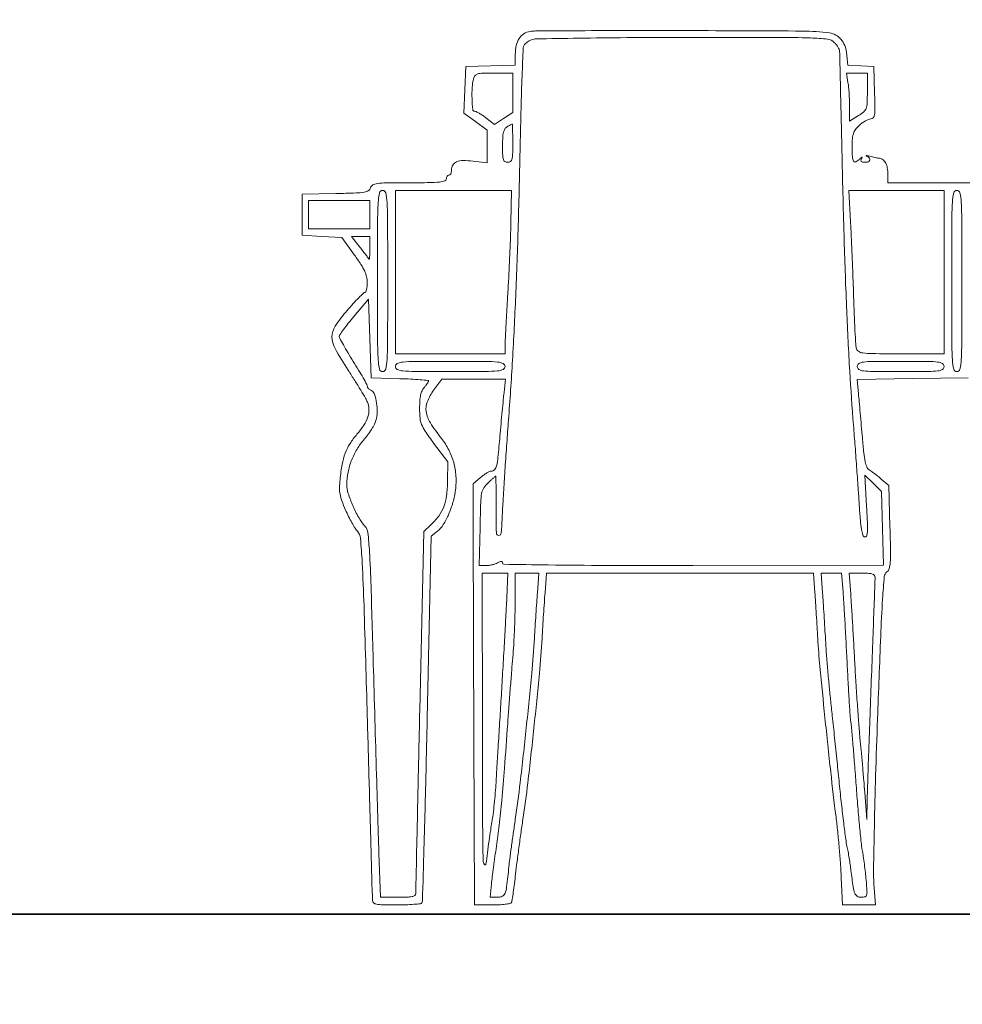
# Model space of a CAD drawing. Units: inches. Extents: x 2416 to 3391, y 1375 to 2496.
# Tile 7 of 13: x 2994 to 3014, y 2142 to 2163. Entities that reach past the tile are written whole.
import ezdxf

# ---------------------------------------------------------------- set-up
doc = ezdxf.new("R2010")
doc.units = ezdxf.units.IN
for name, color, linetype, lineweight in [('A-FLOR-PATT', 252, 'Continuous', 13), ('A-FURN', 8, 'Continuous', 18), ('A-SECT', 7, 'Continuous', 35)]:
    doc.layers.add(name, color=color, linetype=linetype, lineweight=lineweight)

msp = doc.modelspace()

# ---------------------------------------------------------------- hatches: boundary and pattern name
at = {"layer": 'A-FLOR-PATT'}
h = msp.add_hatch(dxfattribs=at)
h.set_pattern_fill('AR-CONC', color=256, scale=0.13, style=0)
h.paths.add_polyline_path([(2904.1924, 2125.8608), (3202.6924, 2125.8608), (3202.6924, 2143.8608), (2904.1924, 2143.8608)])

# ---------------------------------------------------------------- linework, layer by layer
at = {"layer": 'A-FURN'}
msp.add_lwpolyline([(3014.9326, 2159.6193), (3012.3207, 2159.6163), (3012.3199, 2159.796, 0.040694), (3012.3079, 2159.9352, 0.077699), (3012.2724, 2160.0415, 0.104071), (3012.2152, 2160.1115, 0.133976), (3012.1395, 2160.1446, -0.01143), (3012.0998, 2160.1513, -0.004315), (3012.0446, 2160.1625, -0.004271), (3011.9847, 2160.1758, -0.005193), (3011.9289, 2160.1892, 0.008277), (3011.882, 2160.2002, 0.048218), (3011.8569, 2160.2031, 0.677897), (3011.8551, 2160.1988, 0.087429), (3011.8671, 2160.1905, -0.097625), (3011.9225, 2160.1505, -0.27546), (3011.9322, 2160.1057, -0.235276), (3011.8966, 2160.0701, -0.080752), (3011.8226, 2160.0581, -0.041781), (3011.7751, 2160.0621, -0.145697), (3011.7478, 2160.0755, -0.229007), (3011.7392, 2160.0973, -0.110072), (3011.7482, 2160.1268, 0.009535), (3011.7676, 2160.1628, 0.561535), (3011.7644, 2160.1681, 0.184745), (3011.7536, 2160.1639, 0.004358), (3011.713, 2160.1268, -0.07556), (3011.6312, 2160.0712, -0.381609), (3011.5824, 2160.0853, -0.128327), (3011.5562, 2160.1691, -0.012145), (3011.5509, 2160.3858, -0.014739), (3011.5564, 2160.5722, -0.063299), (3011.5769, 2160.6811, -0.086122), (3011.6205, 2160.7643, -0.041944), (3011.7016, 2160.8532, -0.02943), (3011.7665, 2160.9066, -0.029846), (3011.837, 2160.9518, -0.03127), (3011.9028, 2160.9835, -0.096699), (3011.9509, 2160.9929, 0.227876), (3012.0031, 2161.0179, 0.132851), (3012.0314, 2161.0829, 0.039646), (3012.0407, 2161.2215, 0.003895), (3012.034, 2161.5565), (3012.0183, 2162.1201), (3011.7364, 2162.1365), (3011.4544, 2162.1529), (3011.4279, 2162.4293, 0.152427), (3011.3098, 2162.7098, 0.185846), (3011.0619, 2162.846, 0.032345), (3010.4828, 2162.8868, 0.000914), (3007.9886, 2162.8962, 0.000694), (3006.7403, 2162.897, 0.00108), (3005.6642, 2162.8938, 0.000296), (3004.7262, 2162.8884, 0.037431), (3004.6095, 2162.8789, 0.105975), (3004.4761, 2162.8276, 0.106001), (3004.3754, 2162.7261, 0.089007), (3004.3134, 2162.5763, 0.053798), (3004.2927, 2162.3848), (3004.2927, 2162.1516), (3003.7613, 2162.1358), (3003.2298, 2162.1201), (3003.2064, 2161.6185), (3003.1829, 2161.1169), (3003.4354, 2160.9356), (3003.6879, 2160.7543), (3003.6879, 2160.3998), (3003.6879, 2160.0454), (3003.3825, 2160.0836, 0.030857), (3003.166, 2160.0971, 0.100929), (3003.0261, 2160.0687, 0.165736), (3002.9473, 2159.9983, 0.128801), (3002.918, 2159.8864, -0.05129), (3002.914, 2159.8469, -0.071223), (3002.9019, 2159.8135, -0.091278), (3002.884, 2159.791, -0.181272), (3002.8631, 2159.7832, 0.148195), (3002.8421, 2159.7768, 0.098894), (3002.8242, 2159.7589, 0.082425), (3002.8122, 2159.7322, 0.064853), (3002.8081, 2159.7007, -0.329446), (3002.7755, 2159.6567, -0.048884), (3002.6606, 2159.6334, -0.022422), (3002.4464, 2159.621, -0.003188), (3002.0056, 2159.6182, 0.002574), (3001.5111, 2159.6157, 0.029876), (3001.318, 2159.6021, 0.094817), (3001.2217, 2159.5703, 0.204563), (3001.1748, 2159.5098, -0.193942), (3001.13, 2159.4495, -0.096668), (3001.0393, 2159.4157, -0.032405), (3000.8603, 2159.398, -0.003136), (3000.4239, 2159.3861), (2999.7013, 2159.3708), (2999.7013, 2158.9309), (2999.7013, 2158.491), (3000.127, 2158.4635), (3000.5526, 2158.436), (3000.828, 2158.0577, -0.011737), (3000.9673, 2157.8567, -0.036601), (3001.0475, 2157.713, -0.052571), (3001.0893, 2157.5913, -0.056553), (3001.1035, 2157.4666, -0.022205), (3001.0999, 2157.385, -0.035618), (3001.0888, 2157.3163, -0.040242), (3001.0728, 2157.2668, -0.30351), (3001.0534, 2157.2538, 0.194234), (3001.0227, 2157.2414, 0.005517), (3000.9196, 2157.1398, 0.010456), (3000.8004, 2157.0144, 0.00691), (3000.6685, 2156.8657, 0.0303), (3000.4085, 2156.5247, 0.153578), (3000.3419, 2156.2982, 0.122989), (3000.4095, 2156.0476, 0.016581), (3000.6927, 2155.5767, -0.003431), (3000.8333, 2155.3564, -0.004245), (3000.961, 2155.1492, -0.003502), (3001.0655, 2154.9737, -0.031298), (3001.1059, 2154.8936, -0.096896), (3001.139, 2154.7395, -0.083072), (3001.1146, 2154.5752, -0.06581), (3001.0295, 2154.3966, -0.034373), (3000.8811, 2154.1992, 0.037733), (3000.7308, 2153.9965, 0.050819), (3000.6292, 2153.792, 0.04407), (3000.5618, 2153.5496, 0.020527), (3000.5155, 2153.2263, 0.022179), (3000.5051, 2153.0445, 0.048115), (3000.5168, 2152.9052, 0.043671), (3000.5558, 2152.7627, 0.015462), (3000.6354, 2152.5664, 0.011422), (3000.7011, 2152.4265, 0.011589), (3000.7729, 2152.2904, 0.011437), (3000.8407, 2152.175, 0.045753), (3000.8899, 2152.1096, -0.163464), (3000.9561, 2151.9585, -0.008854), (3000.9936, 2151.432, -0.005716), (3001.0327, 2150.4986, -0.000497), (3001.1029, 2148.1231, -0.000065), (3001.1452, 2146.6311, -0.000104), (3001.1809, 2145.3591, -0.000016), (3001.2123, 2144.2298, -0.006771), (3001.2134, 2144.1532, 0.226585), (3001.2376, 2144.1026, 0.124527), (3001.3014, 2144.0733, 0.041075), (3001.4339, 2144.0599, 0.004763), (3001.7326, 2144.057, 0.008183), (3001.9336, 2144.0603, 0.012537), (3002.1075, 2144.0704, 0.007028), (3002.2511, 2144.0843, 0.230516), (3002.2798, 2144.1025, 0.131862), (3002.2918, 2144.1425, 0.000089), (3002.325, 2145.2879, 0.001058), (3002.3591, 2146.5655, 0.000646), (3002.3942, 2148.0741), (3002.4805, 2152.0003), (3002.6157, 2152.1114, 0.081242), (3002.7405, 2152.2535, 0.03703), (3002.856, 2152.4728, 0.034682), (3002.9484, 2152.7327, 0.035128), (3003.0034, 2153.0018, 0.049123), (3003.0133, 2153.2983, 0.050541), (3002.9648, 2153.5882, 0.050681), (3002.8593, 2153.8617, 0.049933), (3002.7006, 2154.1098, -0.026423), (3002.4617, 2154.4472, -0.102499), (3002.3722, 2154.6858, -0.136101), (3002.3974, 2154.9025, -0.061997), (3002.5379, 2155.1535), (3002.7076, 2155.3842), (3003.3941, 2155.3842), (3004.0807, 2155.3842), (3004.0491, 2155.0956, 0.003117), (3004.0333, 2154.9421, 0.000851), (3004.0103, 2154.6996, 0.00086), (3003.9851, 2154.4246, 0.000896), (3003.9612, 2154.1531, -0.003262), (3003.9191, 2153.6991, -0.036009), (3003.888, 2153.5194, -0.119587), (3003.8445, 2153.4359, -0.216199), (3003.7756, 2153.4047, 0.111698), (3003.7384, 2153.3963, 0.023035), (3003.6788, 2153.3644, 0.023156), (3003.6115, 2153.32, 0.019991), (3003.5452, 2153.2675), (3003.3854, 2153.1303), (3003.3854, 2152.209, 0.000667), (3003.3862, 2151.6546, 0.000091), (3003.3895, 2150.4963, 0.000105), (3003.3939, 2149.1241, 0.000088), (3003.3992, 2147.6724), (3003.4129, 2144.057), (3003.7946, 2144.057, 0.011615), (3003.9429, 2144.0605, 0.017148), (3004.0727, 2144.071, 0.012457), (3004.1776, 2144.0857, 0.216373), (3004.2056, 2144.1045, 0.097359), (3004.2192, 2144.1407, 0.003403), (3004.243, 2144.2897, 0.00622), (3004.2679, 2144.4669, 0.004297), (3004.2918, 2144.6681, -0.004039), (3004.3211, 2144.9162, -0.0018), (3004.3636, 2145.2426, -0.001782), (3004.411, 2145.5876, -0.002412), (3004.4565, 2145.8991, 0.008466), (3004.562, 2146.688, 0.002671), (3004.6933, 2147.87, 0.002626), (3004.8114, 2149.0473, 0.009341), (3004.869, 2149.8031, -0.001077), (3004.8834, 2150.0447, -0.000757), (3004.9007, 2150.3166, -0.000764), (3004.9179, 2150.5768, -0.0016), (3004.9323, 2150.7791), (3004.964, 2151.2053), (3007.8393, 2151.2053), (3010.7147, 2151.2053), (3010.7464, 2150.7791, -0.001616), (3010.7607, 2150.5768, -0.000771), (3010.778, 2150.3166, -0.000764), (3010.7952, 2150.0447, -0.001088), (3010.8096, 2149.8031, 0.009311), (3010.8559, 2149.1931, 0.001798), (3010.9643, 2148.0916, 0.002045), (3011.0886, 2146.921, 0.00359), (3011.2023, 2145.954, -0.005555), (3011.2383, 2145.6373, -0.003761), (3011.2725, 2145.2756, -0.003789), (3011.3004, 2144.9255, -0.007555), (3011.3161, 2144.6481), (3011.3407, 2144.057), (3011.6982, 2144.057), (3012.0557, 2144.057), (3012.0202, 2144.5106, -0.023542), (3012.0107, 2144.8164, -0.001398), (3012.0282, 2145.7418, -0.002102), (3012.0568, 2146.844, -0.001549), (3012.0973, 2148.0646, -0.000733), (3012.1647, 2149.8479, -0.006199), (3012.2061, 2150.6501, -0.006766), (3012.2435, 2151.1307, -0.215322), (3012.3003, 2151.2311, 0.172904), (3012.3488, 2151.3024, 0.046951), (3012.3709, 2151.439, 0.021167), (3012.3769, 2151.6806, 0.002768), (3012.3649, 2152.1946), (3012.339, 2153.0921), (3012.1739, 2153.2346, 0.007641), (3012.1039, 2153.2933, 0.006997), (3012.0301, 2153.3515, 0.007013), (3011.9628, 2153.4016, 0.02266), (3011.9161, 2153.4322, -0.164534), (3011.8671, 2153.4893, -0.043552), (3011.8315, 2153.6059, -0.025507), (3011.8012, 2153.7957, -0.005821), (3011.7702, 2154.1195, 0.000569), (3011.7476, 2154.3848, 0.000516), (3011.7236, 2154.6587, 0.000516), (3011.7017, 2154.9038, 0.001658), (3011.6863, 2155.067), (3011.6557, 2155.3821), (3012.8543, 2155.3969), (3014.0528, 2155.4117)], format="xyb", dxfattribs=at)
for points in [[(3011.166, 2162.6425, -0.026778), (3011.2084, 2162.5953, -0.028055), (3011.2447, 2162.5446, -0.029182), (3011.2709, 2162.4975, -0.099615), (3011.2796, 2162.4638, -0.007318), (3011.2816, 2162.4095, -0.000026), (3011.2963, 2161.7691, -0.000141), (3011.3127, 2161.0437, -0.000089), (3011.3315, 2160.1956, 0.001893), (3011.3785, 2158.3755, 0.00325), (3011.4332, 2156.8588, 0.003838), (3011.4987, 2155.5561, 0.005389), (3011.5786, 2154.3945, -0.00099), (3011.6142, 2153.9359, -0.000806), (3011.6505, 2153.4447, -0.000814), (3011.6826, 2152.9921, -0.002127), (3011.7037, 2152.6668, 0.005605), (3011.7267, 2152.3468, 0.021905), (3011.7517, 2152.1501, 0.031188), (3011.781, 2152.0267, 0.24354), (3011.821, 2151.9857, 0.404876), (3011.8594, 2152.0043, 0.072476), (3011.8775, 2152.0902, 0.025662), (3011.8795, 2152.2671, 0.003415), (3011.862, 2152.6403), (3011.8254, 2153.3206), (3012.0036, 2153.1424), (3012.1818, 2152.9642), (3012.2023, 2152.1698), (3012.2229, 2151.3754), (3008.1203, 2151.3716, -0.000826), (3006.2417, 2151.373, -0.002714), (3005.0015, 2151.3827, -0.000471), (3004.047, 2151.3963, -0.409789), (3004.0178, 2151.426, 0.166213), (3004.0104, 2151.4476, 0.22914), (3003.9923, 2151.4565, 0.10154), (3003.9604, 2151.4504, 0.024401), (3003.9114, 2151.4271, -0.043973), (3003.8603, 2151.4053, -0.023243), (3003.7937, 2151.3869, -0.022945), (3003.7233, 2151.3744, -0.032736), (3003.66, 2151.3702), (3003.515, 2151.3702), (3003.5327, 2152.1899, -0.002627), (3003.5472, 2152.7296, -0.036146), (3003.5676, 2152.9242, -0.096216), (3003.6129, 2153.0418, -0.065991), (3003.7044, 2153.1521, -0.003279), (3003.7643, 2153.2068, -0.005161), (3003.8164, 2153.2529, -0.00157), (3003.862, 2153.2921, -0.176898), (3003.8694, 2153.2948, -0.410724), (3003.8739, 2153.2905, -0.000294), (3003.8771, 2153.1092, -0.002699), (3003.8795, 2152.9052, -0.001618), (3003.8803, 2152.6629, 0.003665), (3003.8846, 2152.0706, 0.408936), (3003.9357, 2152.0201, 0.396408), (3003.9893, 2152.0702, 0.00365), (3004.0233, 2152.6624, -0.00305), (3004.042, 2152.996, -0.001065), (3004.0729, 2153.4757, -0.001058), (3004.1091, 2154.0035, -0.001235), (3004.1458, 2154.5045, 0.004548), (3004.2317, 2155.7945, 0.003739), (3004.3006, 2157.1729, 0.003361), (3004.355, 2158.6944, 0.002316), (3004.397, 2160.4189, -0.001849), (3004.416, 2161.2262, -0.002933), (3004.4388, 2161.9173, -0.000677), (3004.4631, 2162.5223, -0.128702), (3004.4811, 2162.581, -0.068231), (3004.5058, 2162.6109, -0.029137), (3004.546, 2162.6438, -0.028159), (3004.5936, 2162.6745, -0.033036), (3004.642, 2162.6978, -0.091686), (3004.7375, 2162.7172, -0.000531), (3005.6501, 2162.7325, -0.002226), (3006.6929, 2162.7442, -0.001411), (3007.9081, 2162.7489, -0.000515), (3009.9481, 2162.7491, -0.007931), (3010.6506, 2162.7373, -0.018651), (3011.0223, 2162.7112, -0.171176)], [(3004.237, 2161.5565), (3004.2364, 2161.1303), (3004.0403, 2161.0033), (3003.8443, 2160.8763), (3003.6598, 2161.0171, 0.014107), (3003.5848, 2161.071, 0.01763), (3003.5122, 2161.1165, 0.015997), (3003.4496, 2161.1501, 0.115683), (3003.4166, 2161.1578, -0.387752), (3003.3746, 2161.1962, -0.014242), (3003.3599, 2161.43, -0.023123), (3003.3628, 2161.6746, -0.050938), (3003.3926, 2161.8589, -0.105762), (3003.4274, 2161.9269, -0.154427), (3003.4832, 2161.9636, -0.06207), (3003.5873, 2161.9794, -0.006663), (3003.8317, 2161.9826), (3004.2377, 2161.9826)], [(3011.8785, 2161.584, -0.008054), (3011.8729, 2161.3271, -0.079294), (3011.8518, 2161.2213, -0.129075), (3011.8011, 2161.1489, -0.033836), (3011.6861, 2161.0641), (3011.4959, 2160.9429), (3011.4953, 2161.2566, 0.009103), (3011.4926, 2161.3918, 0.007073), (3011.4849, 2161.5387, 0.007158), (3011.4738, 2161.6755, 0.017138), (3011.4606, 2161.7764), (3011.4266, 2161.9826), (3011.6537, 2161.9826), (3011.8808, 2161.9826)], [(3004.2377, 2160.4705, -0.005909), (3004.2348, 2160.2248, -0.059311), (3004.2203, 2160.1234, -0.180365), (3004.1868, 2160.0763, -0.150217), (3004.1277, 2160.0581, -0.133688), (3004.0692, 2160.074, -0.18676), (3004.0358, 2160.1162, -0.067763), (3004.0209, 2160.2054, -0.007506), (3004.0178, 2160.4128, -0.01155), (3004.022, 2160.5955, -0.046016), (3004.0374, 2160.7065, -0.080745), (3004.0666, 2160.7773, -0.123363), (3004.114, 2160.8235, -0.004566), (3004.1519, 2160.8451, -0.006456), (3004.186, 2160.8636, -0.003906), (3004.215, 2160.8785, -0.086883), (3004.224, 2160.8812, -0.43878), (3004.2296, 2160.8764, -0.001111), (3004.2337, 2160.7613, -0.00524), (3004.2367, 2160.6285, -0.003124)], [(3001.5434, 2157.5012, -0.000789), (3001.5414, 2156.2278, -0.013281), (3001.5289, 2155.8069, -0.040964), (3001.5005, 2155.6029, -0.351139), (3001.4334, 2155.5492, -0.351139), (3001.3663, 2155.6029, -0.040964), (3001.3379, 2155.8069, -0.013281), (3001.3254, 2156.2278, -0.000789), (3001.3234, 2157.5012, -0.000789), (3001.3254, 2158.7746, -0.013281), (3001.3379, 2159.1955, -0.040964), (3001.3663, 2159.3995, -0.351139), (3001.4334, 2159.4532, -0.351139), (3001.5005, 2159.3995, -0.040964), (3001.5289, 2159.1955, -0.013281), (3001.5414, 2158.7746, -0.000789)], [(3004.1965, 2158.7522, -0.004002), (3004.1873, 2158.4209, -0.001949), (3004.1706, 2157.9982, -0.001933), (3004.1498, 2157.5584, -0.002793), (3004.1277, 2157.1698, 0.001149), (3004.1067, 2156.8194, 0.001454), (3004.0889, 2156.4954, 0.001145), (3004.0754, 2156.2235, 0.01183), (3004.0728, 2156.1113), (3004.0728, 2155.9341), (3002.8905, 2155.9341), (3001.7083, 2155.9341), (3001.7083, 2157.6937), (3001.7083, 2159.4532), (3002.9593, 2159.4533), (3004.2102, 2159.4534)], [(3013.5304, 2157.6909), (3013.5304, 2155.9341), (3012.5967, 2155.9341, -0.001796), (3011.9824, 2155.9363, -0.030294), (3011.78, 2155.95, -0.119585), (3011.6849, 2155.9865, -0.193912), (3011.6379, 2156.0578, -0.035598), (3011.6268, 2156.1435, -0.001758), (3011.6113, 2156.4279, -0.002835), (3011.596, 2156.7662, -0.002044), (3011.5826, 2157.1438, 0.001345), (3011.5683, 2157.5613, 0.001011), (3011.5505, 2158.0206, 0.001022), (3011.532, 2158.4525, 0.002353), (3011.5159, 2158.7772), (3011.4794, 2159.4484), (3012.5049, 2159.448), (3013.5304, 2159.4476)], [(3013.9153, 2157.5012, -0.000789), (3013.9133, 2156.2278, -0.013281), (3013.9008, 2155.8069, -0.040964), (3013.8725, 2155.6029, -0.351139), (3013.8054, 2155.5492, -0.351139), (3013.7383, 2155.6029, -0.040964), (3013.7099, 2155.8069, -0.013281), (3013.6974, 2156.2278, -0.000789), (3013.6954, 2157.5012, -0.000789), (3013.6974, 2158.7746, -0.013281), (3013.7099, 2159.1955, -0.040964), (3013.7383, 2159.3995, -0.351139), (3013.8054, 2159.4532, -0.351139), (3013.8725, 2159.3995, -0.040964), (3013.9008, 2159.1955, -0.013281), (3013.9133, 2158.7746, -0.000789)], [(3001.1585, 2158.2069, -0.006182), (3001.1573, 2158.11, -0.011852), (3001.1535, 2158.0324, -0.009529), (3001.1483, 2157.975, -0.682734), (3001.1416, 2157.9732, 0.004799), (3001.1293, 2157.9895, 0.00014), (3001.0767, 2158.058, 0.000282), (3001.0148, 2158.1386, 0.000194), (3000.9445, 2158.2298), (3000.7643, 2158.4635), (3000.9614, 2158.4635), (3001.1585, 2158.4635)], [(3001.8046, 2155.3962, -0.005316), (3002.0418, 2155.3877, -0.008829), (3002.2414, 2155.3749, -0.003101), (3002.41, 2155.36, -0.38691), (3002.4232, 2155.3455, -0.132522), (3002.4179, 2155.326, -0.0176), (3002.3949, 2155.2895, -0.019379), (3002.3638, 2155.2474, -0.015163), (3002.3269, 2155.2041, 0.079783), (3002.2822, 2155.1352, 0.051249), (3002.2526, 2155.0445, 0.037499), (3002.2359, 2154.9231, 0.015592), (3002.2307, 2154.7576, 0.022364), (3002.2402, 2154.5444, 0.073811), (3002.2732, 2154.408, 0.054883), (3002.3491, 2154.2669, 0.008594), (3002.5331, 2154.0095), (3002.8356, 2153.6015), (3002.8325, 2153.1869, -0.030332), (3002.8114, 2152.8774, -0.059146), (3002.751, 2152.6377, -0.065957), (3002.6418, 2152.4362, -0.047783), (3002.4724, 2152.2447), (3002.3181, 2152.1005), (3002.2332, 2148.2408, 0.000042), (3002.2006, 2146.7554, 0.000069), (3002.1732, 2145.4915, 0.000009), (3002.1489, 2144.3653, 0.00538), (3002.1482, 2144.3015, -0.251891), (3002.1275, 2144.263, -0.094475), (3002.069, 2144.2386, -0.042833), (3001.9607, 2144.2254, -0.008939), (3001.7692, 2144.222), (3001.3902, 2144.222), (3001.3551, 2145.1705, -0.00149), (3001.3365, 2145.714, -0.000272), (3001.3058, 2146.7204, -0.000292), (3001.2711, 2147.8984, -0.000265), (3001.2366, 2149.1149, 0.000675), (3001.1837, 2150.9304, 0.007217), (3001.1506, 2151.6675, 0.012531), (3001.1156, 2152.0813, 0.159182), (3001.052, 2152.2217, -0.055674), (3000.9187, 2152.4046, -0.027511), (3000.7901, 2152.662, -0.027162), (3000.693, 2152.9248, -0.075092), (3000.6636, 2153.1192, -0.048065), (3000.6886, 2153.3787, -0.044181), (3000.7628, 2153.6365, -0.04369), (3000.8822, 2153.8799, -0.044634), (3001.0414, 2154.0971, 0.024929), (3001.1301, 2154.2086, 0.022668), (3001.2103, 2154.3319, 0.023372), (3001.272, 2154.449, 0.063213), (3001.3007, 2154.5382, 0.050059), (3001.3167, 2154.7247, 0.044267), (3001.2966, 2154.9188, 0.045765), (3001.25, 2155.079, 0.210498), (3001.1829, 2155.1456, -0.057858), (3001.1525, 2155.1615, -0.058904), (3001.1268, 2155.1838, -0.065001), (3001.1093, 2155.2089, -0.12013), (3001.1035, 2155.233, 0.125186), (3001.0938, 2155.271, 0.003848), (3001.0146, 2155.4139, 0.007344), (3000.9169, 2155.5814, 0.004991), (3000.8011, 2155.7691, -0.00512), (3000.6852, 2155.957, -0.007511), (3000.5875, 2156.1248, -0.004013), (3000.5085, 2156.2679, -0.124719), (3000.4986, 2156.3068, -0.153596), (3000.5102, 2156.3436, -0.006383), (3000.5915, 2156.4569, -0.010547), (3000.6937, 2156.5896, -0.007244), (3000.8148, 2156.7358), (3001.131, 2157.1064), (3001.1585, 2156.2591), (3001.186, 2155.4117)], [(3004.0728, 2155.6592, -0.295956), (3004.0316, 2155.5958, -0.08195), (3003.9112, 2155.5642, -0.021776), (3003.6498, 2155.5513, -0.001417), (3002.8905, 2155.5492, -0.001417), (3002.1313, 2155.5513, -0.021776), (3001.8699, 2155.5642, -0.08195), (3001.7495, 2155.5958, -0.295956), (3001.7083, 2155.6592, -0.295956), (3001.7495, 2155.7226, -0.08195), (3001.8699, 2155.7541, -0.021776), (3002.1313, 2155.767, -0.001417), (3002.8905, 2155.7691, -0.001417), (3003.6498, 2155.767, -0.021776), (3003.9112, 2155.7541, -0.08195), (3004.0316, 2155.7226, -0.295956)], [(3013.5304, 2155.6592, -0.263491), (3013.4953, 2155.5971, -0.106183), (3013.3999, 2155.5646, -0.027391), (3013.1898, 2155.5514, -0.001893), (3012.5957, 2155.5492, -0.001893), (3012.0016, 2155.5514, -0.027391), (3011.7915, 2155.5646, -0.106183), (3011.696, 2155.5971, -0.263491), (3011.6609, 2155.6592, -0.263491), (3011.696, 2155.7212, -0.106183), (3011.7915, 2155.7538, -0.027391), (3012.0016, 2155.7669, -0.001893), (3012.5957, 2155.7691, -0.001893), (3013.1898, 2155.7669, -0.027391), (3013.3999, 2155.7538, -0.106183), (3013.4953, 2155.7212, -0.263491)], [(3004.0996, 2150.5042, -0.001601), (3004.0815, 2150.1477, -0.000544), (3004.0529, 2149.6295, -0.00054), (3004.02, 2149.057, -0.000622), (3003.9874, 2148.5109, 0.000055), (3003.9549, 2147.9779, 0.000055), (3003.9226, 2147.4449, 0.000053), (3003.8945, 2146.9795, 0.000217), (3003.8775, 2146.6964, -0.00616), (3003.8614, 2146.4722, -0.00489), (3003.8387, 2146.2305, -0.004946), (3003.8132, 2146.0068, -0.012329), (3003.789, 2145.8441, 0.005904), (3003.762, 2145.678, 0.002132), (3003.7275, 2145.4415, 0.002114), (3003.6919, 2145.182, 0.002512), (3003.6606, 2144.9368, -0.685021), (3003.6286, 2144.9287, -0.148627), (3003.6004, 2145.0132, -0.005875), (3003.5891, 2145.7535, -0.000433), (3003.5838, 2147.7823), (3003.5779, 2151.2053), (3003.8555, 2151.2053), (3004.1331, 2151.2053)], [(3004.7673, 2150.7791, 0.0016), (3004.753, 2150.5768, 0.000764), (3004.7357, 2150.3166, 0.000757), (3004.7185, 2150.0447, 0.001077), (3004.7041, 2149.8031, -0.009332), (3004.6468, 2149.0519, -0.002583), (3004.5289, 2147.875, -0.002638), (3004.3978, 2146.6919, -0.008272), (3004.2924, 2145.8991, 0.001676), (3004.2491, 2145.6032, 0.001648), (3004.2075, 2145.3054, 0.001619), (3004.1727, 2145.044, 0.006283), (3004.1538, 2144.8818, -0.003757), (3004.1056, 2144.4508, -0.059536), (3004.0709, 2144.3078, -0.198332), (3004.0125, 2144.2449, -0.108152), (3003.9079, 2144.222), (3003.748, 2144.222), (3003.7781, 2144.5106, -0.005194), (3003.7948, 2144.6569, -0.001789), (3003.822, 2144.868, -0.001778), (3003.8537, 2145.1005, -0.00206), (3003.8855, 2145.3217, 0.00865), (3003.9443, 2145.7724, 0.005187), (3003.9993, 2146.3094, 0.003824), (3004.0577, 2147.0029, 0.001495), (3004.1281, 2147.9611, -0.000898), (3004.1548, 2148.3296, -0.000687), (3004.1852, 2148.7326, -0.000695), (3004.2148, 2149.1098, -0.001643), (3004.2381, 2149.3907, 0.00681), (3004.2574, 2149.6564, 0.003803), (3004.274, 2149.9802, 0.003793), (3004.2858, 2150.3079, 0.006149), (3004.2903, 2150.5867), (3004.2927, 2151.2053), (3004.5459, 2151.2053), (3004.799, 2151.2053)], [(3011.3537, 2150.8066, -0.004862), (3011.3696, 2150.5826, -0.000992), (3011.393, 2150.1859, -0.001045), (3011.4184, 2149.7246, -0.00098), (3011.4424, 2149.2532, 0.001439), (3011.4657, 2148.8028, 0.002089), (3011.4891, 2148.4054, 0.001048), (3011.5111, 2148.0682, 0.035374), (3011.5222, 2147.9885, -0.030177), (3011.5341, 2147.9087, -0.000856), (3011.564, 2147.5636, -0.00174), (3011.597, 2147.1573, -0.001195), (3011.6317, 2146.6964, 0.002298), (3011.6684, 2146.2236, 0.002787), (3011.7073, 2145.7807, 0.002356), (3011.7438, 2145.4084, 0.019242), (3011.7678, 2145.2392, -0.008848), (3011.7893, 2145.1076, -0.004103), (3011.8128, 2144.936, -0.004063), (3011.8345, 2144.7553, -0.005647), (3011.8508, 2144.5931, -0.004997), (3011.87, 2144.3501, -0.08419), (3011.8621, 2144.2702, -0.254544), (3011.8273, 2144.234, -0.076835), (3011.7493, 2144.222, -0.130915), (3011.6611, 2144.2455, -0.171535), (3011.6071, 2144.3082, -0.057608), (3011.5712, 2144.4458, -0.005199), (3011.525, 2144.7993, 0.006659), (3011.5085, 2144.9226, 0.004184), (3011.4861, 2145.0662, 0.004199), (3011.4617, 2145.2072, 0.007668), (3011.4391, 2145.3217, -0.019768), (3011.4126, 2145.4751, -0.00232), (3011.3687, 2145.8195, -0.002778), (3011.3207, 2146.2297, -0.002271), (3011.2738, 2146.6689, 0.00026), (3011.2251, 2147.1423, 0.000204), (3011.1719, 2147.6555, 0.000206), (3011.122, 2148.1329, 0.000508), (3011.0848, 2148.4834, -0.003349), (3011.0532, 2148.7992, -0.002298), (3011.0213, 2149.1579, -0.002316), (3010.9938, 2149.5035, -0.004705), (3010.976, 2149.7756, 0.001171), (3010.9613, 2150.0278, 0.000849), (3010.9437, 2150.3085, 0.000858), (3010.9262, 2150.575, 0.001876), (3010.9116, 2150.7791), (3010.8796, 2151.2053), (3011.1006, 2151.2053), (3011.3216, 2151.2053)], [(3012.0444, 2151.109, -0.005402), (3012.0425, 2151.0347, -0.00004), (3012.02, 2150.4192, -0.000151), (3011.9939, 2149.7142, -0.000097), (3011.9633, 2148.8958, 0.000323), (3011.9322, 2148.053, 0.000406), (3011.9044, 2147.2715, 0.000324), (3011.8821, 2146.6156, 0.003186), (3011.8746, 2146.3389), (3011.8655, 2145.8991), (3011.8218, 2146.4764, 0.00174), (3011.8008, 2146.7411, 0.000983), (3011.7736, 2147.0618, 0.000981), (3011.7449, 2147.3852, 0.001613), (3011.7192, 2147.6586, -0.005024), (3011.6929, 2147.9605, -0.001879), (3011.6619, 2148.3846, -0.001862), (3011.6315, 2148.8469, -0.002256), (3011.6066, 2149.2807, 0.000812), (3011.5836, 2149.7035, 0.000777), (3011.5588, 2150.1324, 0.000769), (3011.5358, 2150.511, 0.002791), (3011.5194, 2150.7516), (3011.4861, 2151.2053), (3011.7659, 2151.2053, -0.01208), (3011.9153, 2151.2016, -0.071226), (3011.992, 2151.1869, -0.165066), (3012.0303, 2151.1571, -0.15076)]]:
    msp.add_lwpolyline(points, format="xyb", close=True, dxfattribs=at)
msp.add_lwpolyline([(3001.1585, 2158.9309), (3001.1585, 2158.6284), (3000.4986, 2158.6284), (2999.8388, 2158.6284), (2999.8388, 2158.9309), (2999.8388, 2159.2333), (3000.4986, 2159.2333), (3001.1585, 2159.2333)], close=True, dxfattribs=at)
at = {"layer": 'A-SECT'}
msp.add_line((3202.6924, 2143.8608), (2904.1924, 2143.8608), dxfattribs=at)

doc.saveas('drawing.dxf')
